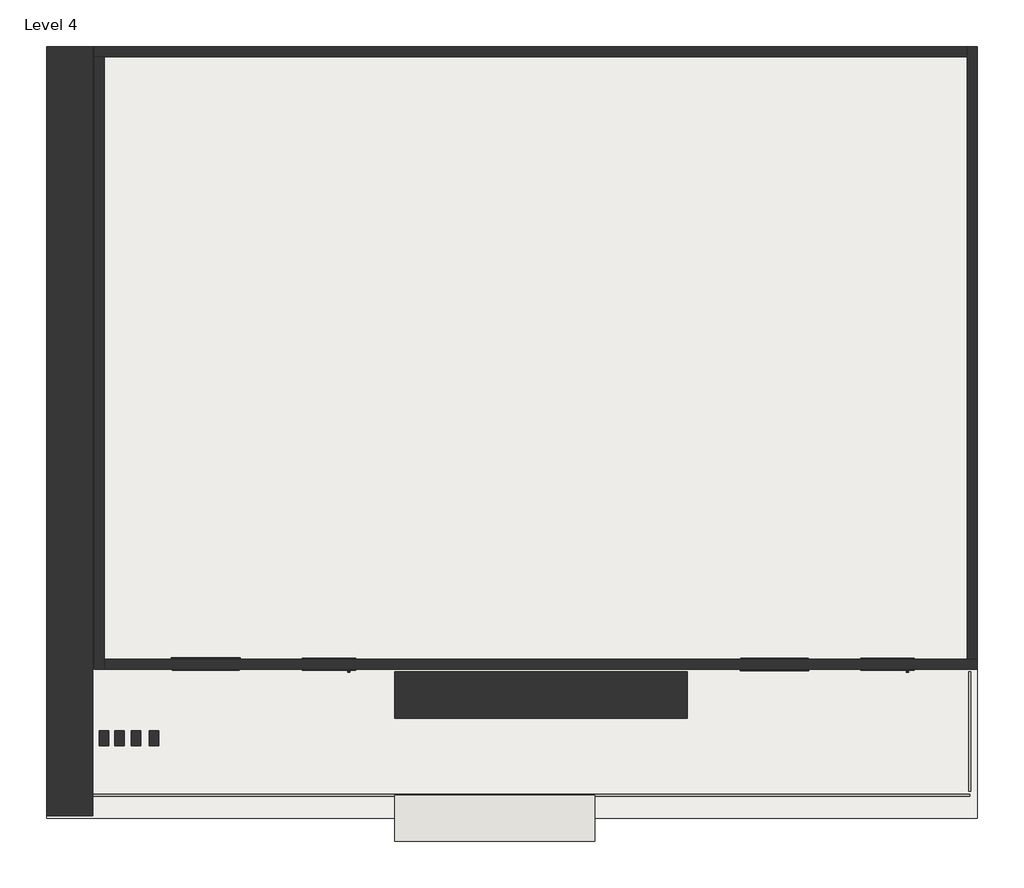
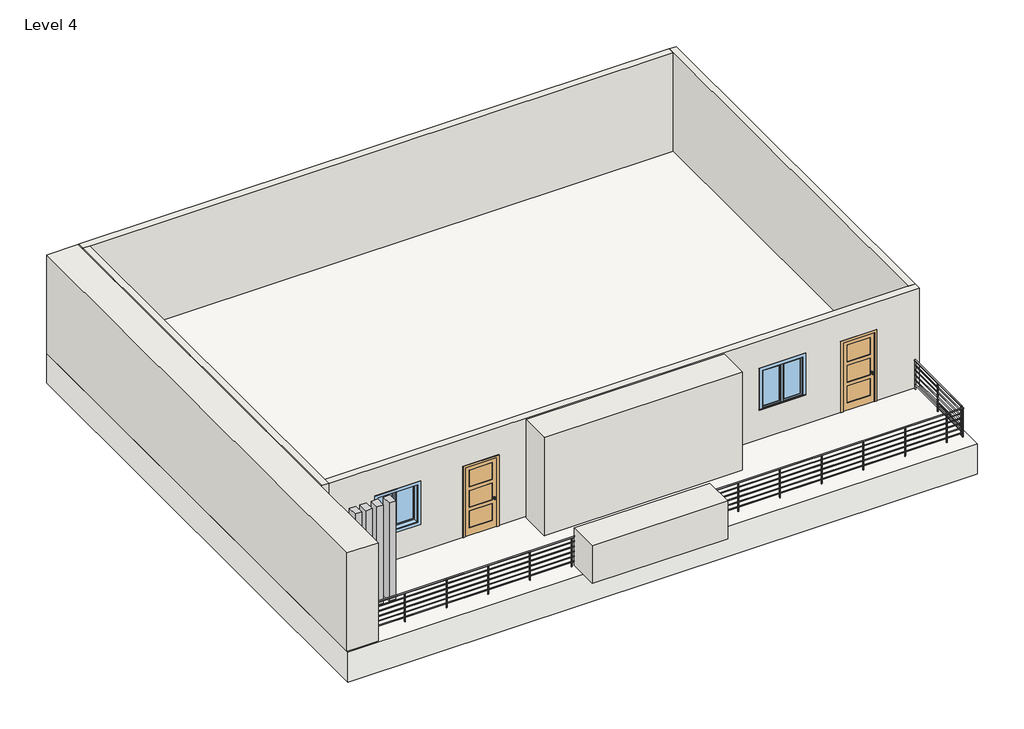
# One storey: 7 walls, 4 columns, 2 doors, 2 railings, 2 windows, 1 slab.
"""IFC4 building model written with IfcOpenShell, lengths in millimetres."""

from ifc_helpers import new_model, si_unit, point, frame, frame_2d, origin, place, context, project, spatial, polyline, circle_curve, trimmed, segment, composite_curve, outline, extrude, faceted_brep, transform, mapped, element, save
from components import wood_timber_column_8_x_12_853526f8, door_54d869bf, window_3a1167bf, window_0862ab64

model = new_model("IFC4")

# Units and contexts
model_context = context("Model", 3, world=origin())
ifc_project = project(units=[si_unit("LENGTHUNIT", "METRE", prefix="MILLI")], contexts=[model_context])

# Site, building, storey
site = spatial("IfcSite", under=ifc_project)
building = spatial("IfcBuilding", under=site)
storey = spatial("IfcBuildingStorey", under=building, Name="Level 4", Elevation=9144.0)

# Columns
placement = place(None, origin())
wood_timber_column_8_x_12_shape = wood_timber_column_8_x_12_853526f8(model_context)
element("IfcColumn", 1, ObjectType="Wood Timber Column : 8 x 12", at=placement, inside=storey, context=model_context, shape_type="MappedRepresentation", body=[
    mapped(wood_timber_column_8_x_12_shape, transform((-18270.7121948, 4590.8323495, 0.0), x_axis=(1.0, 0.0, 0.0), y_axis=(0.0, 1.0, 0.0), z_axis=(0.0, 0.0, 1.0))),
])
element("IfcColumn", 2, ObjectType="Wood Timber Column : 8 x 12", at=placement, inside=storey, context=model_context, shape_type="MappedRepresentation", body=[
    mapped(wood_timber_column_8_x_12_shape, transform((-18600.9121948, 4590.8323495, 0.0), x_axis=(1.0, 0.0, 0.0), y_axis=(0.0, 1.0, 0.0), z_axis=(0.0, 0.0, 1.0))),
])
element("IfcColumn", 3, ObjectType="Wood Timber Column : 8 x 12", at=placement, inside=storey, context=model_context, shape_type="MappedRepresentation", body=[
    mapped(wood_timber_column_8_x_12_shape, transform((-18905.7121948, 4590.8323495, 0.0), x_axis=(1.0, 0.0, 0.0), y_axis=(0.0, 1.0, 0.0), z_axis=(0.0, 0.0, 1.0))),
])
element("IfcColumn", 4, ObjectType="Wood Timber Column : 8 x 12", at=placement, inside=storey, context=model_context, shape_type="MappedRepresentation", body=[
    mapped(wood_timber_column_8_x_12_shape, transform((-17915.1121948, 4590.8323495, 0.0), x_axis=(1.0, 0.0, 0.0), y_axis=(0.0, 1.0, 0.0), z_axis=(0.0, 0.0, 1.0))),
])

# Doors
door_shape = door_54d869bf(model_context)
element("IfcDoor", 5, ObjectType="Door-Interior-Single-3_Panel_Vert-Wood : 36\" x 84\" 2", at=placement, inside=storey, context=model_context, shape_type="MappedRepresentation", body=[
    mapped(door_shape, transform((-3405.3621948, 6054.574368, 7844.0883406), x_axis=(-1.0, 0.0, 0.0), y_axis=(0.0, -1.0, 0.0), z_axis=(0.0, 0.0, 1.0))),
])
element("IfcDoor", 6, ObjectType="Door-Interior-Single-3_Panel_Vert-Wood : 36\" x 84\" 2", at=placement, inside=storey, context=model_context, shape_type="MappedRepresentation", body=[
    mapped(door_shape, transform((-14454.3621948, 6054.574368, 7844.0883406), x_axis=(-1.0, 0.0, 0.0), y_axis=(0.0, -1.0, 0.0), z_axis=(0.0, 0.0, 1.0))),
])

# Railings
element("IfcRailing", 7, ObjectType="Handrail - Pipe", at=placement, inside=storey, context=model_context, shape_type="SweptSolid", body=[
    extrude(outline(composite_curve([segment(trimmed(circle_curve(frame_2d((3466.949368, 8739.4383406)), 19.05), [point((3447.899368, 8739.4383406))], [point((3485.999368, 8739.4383406))], False, "CARTESIAN"), True, "CONTINUOUS"), segment(trimmed(circle_curve(frame_2d((3466.949368, 8739.4383406)), 19.05), [point((3485.999368, 8739.4383406))], [point((3447.899368, 8739.4383406))], False, "CARTESIAN"), True, "CONTINUOUS")], self_intersect=False)), frame((-19331.1621948, 0.0, 0.0), z_axis=(1.0, 0.0, 0.0), x_axis=(0.0, 1.0, 0.0)), (0.0, 0.0, 1.0), 17551.4),
    extrude(outline(composite_curve([segment(trimmed(circle_curve(frame_2d((3466.949368, 8593.3883406)), 12.7), [point((3479.649368, 8593.3883406))], [point((3454.249368, 8593.3883406))], False, "CARTESIAN"), True, "CONTINUOUS"), segment(trimmed(circle_curve(frame_2d((3466.949368, 8593.3883406)), 12.7), [point((3454.249368, 8593.3883406))], [point((3479.649368, 8593.3883406))], False, "CARTESIAN"), True, "CONTINUOUS")], self_intersect=False)), frame((-19331.1621948, 0.0, 0.0), z_axis=(1.0, 0.0, 0.0), x_axis=(0.0, 1.0, 0.0)), (0.0, 0.0, 1.0), 17551.4),
    extrude(outline(composite_curve([segment(trimmed(circle_curve(frame_2d((3466.949368, 8440.9883406)), 12.7), [point((3479.649368, 8440.9883406))], [point((3454.249368, 8440.9883406))], False, "CARTESIAN"), True, "CONTINUOUS"), segment(trimmed(circle_curve(frame_2d((3466.949368, 8440.9883406)), 12.7), [point((3454.249368, 8440.9883406))], [point((3479.649368, 8440.9883406))], False, "CARTESIAN"), True, "CONTINUOUS")], self_intersect=False)), frame((-19331.1621948, 0.0, 0.0), z_axis=(1.0, 0.0, 0.0), x_axis=(0.0, 1.0, 0.0)), (0.0, 0.0, 1.0), 17551.4),
    extrude(outline(composite_curve([segment(trimmed(circle_curve(frame_2d((3466.949368, 8288.5883406)), 12.7), [point((3479.649368, 8288.5883406))], [point((3454.249368, 8288.5883406))], False, "CARTESIAN"), True, "CONTINUOUS"), segment(trimmed(circle_curve(frame_2d((3466.949368, 8288.5883406)), 12.7), [point((3454.249368, 8288.5883406))], [point((3479.649368, 8288.5883406))], False, "CARTESIAN"), True, "CONTINUOUS")], self_intersect=False)), frame((-19331.1621948, 0.0, 0.0), z_axis=(1.0, 0.0, 0.0), x_axis=(0.0, 1.0, 0.0)), (0.0, 0.0, 1.0), 17551.4),
    extrude(outline(composite_curve([segment(trimmed(circle_curve(frame_2d((3466.949368, 8136.1883406)), 12.7), [point((3479.649368, 8136.1883406))], [point((3454.249368, 8136.1883406))], False, "CARTESIAN"), True, "CONTINUOUS"), segment(trimmed(circle_curve(frame_2d((3466.949368, 8136.1883406)), 12.7), [point((3454.249368, 8136.1883406))], [point((3479.649368, 8136.1883406))], False, "CARTESIAN"), True, "CONTINUOUS")], self_intersect=False)), frame((-19331.1621948, 0.0, 0.0), z_axis=(1.0, 0.0, 0.0), x_axis=(0.0, 1.0, 0.0)), (0.0, 0.0, 1.0), 17551.4),
    extrude(outline(composite_curve([segment(trimmed(circle_curve(frame_2d((3466.949368, 7983.7883406)), 12.7), [point((3479.649368, 7983.7883406))], [point((3454.249368, 7983.7883406))], False, "CARTESIAN"), True, "CONTINUOUS"), segment(trimmed(circle_curve(frame_2d((3466.949368, 7983.7883406)), 12.7), [point((3454.249368, 7983.7883406))], [point((3479.649368, 7983.7883406))], False, "CARTESIAN"), True, "CONTINUOUS")], self_intersect=False)), frame((-19331.1621948, 0.0, 0.0), z_axis=(1.0, 0.0, 0.0), x_axis=(0.0, 1.0, 0.0)), (0.0, 0.0, 1.0), 17551.4),
    extrude(outline(composite_curve([segment(trimmed(circle_curve(frame_2d((-2262.3621948, 3466.949368)), 12.7), [point((-2262.3621948, 3479.649368))], [point((-2262.3621948, 3454.249368))], False, "CARTESIAN"), True, "CONTINUOUS"), segment(trimmed(circle_curve(frame_2d((-2262.3621948, 3466.949368)), 12.7), [point((-2262.3621948, 3454.249368))], [point((-2262.3621948, 3479.649368))], False, "CARTESIAN"), True, "CONTINUOUS")], self_intersect=False)), frame((0.0, 0.0, 7844.0883406), z_axis=(0.0, 0.0, 1.0), x_axis=(1.0, 0.0, 0.0)), (0.0, 0.0, 1.0), 876.3),
    extrude(outline(composite_curve([segment(trimmed(circle_curve(frame_2d((-3481.5621948, 3466.949368)), 12.7), [point((-3481.5621948, 3479.649368))], [point((-3481.5621948, 3454.249368))], False, "CARTESIAN"), True, "CONTINUOUS"), segment(trimmed(circle_curve(frame_2d((-3481.5621948, 3466.949368)), 12.7), [point((-3481.5621948, 3454.249368))], [point((-3481.5621948, 3479.649368))], False, "CARTESIAN"), True, "CONTINUOUS")], self_intersect=False)), frame((0.0, 0.0, 7844.0883406), z_axis=(0.0, 0.0, 1.0), x_axis=(1.0, 0.0, 0.0)), (0.0, 0.0, 1.0), 876.3),
    extrude(outline(composite_curve([segment(trimmed(circle_curve(frame_2d((-4700.7621948, 3466.949368)), 12.7), [point((-4700.7621948, 3479.649368))], [point((-4700.7621948, 3454.249368))], False, "CARTESIAN"), True, "CONTINUOUS"), segment(trimmed(circle_curve(frame_2d((-4700.7621948, 3466.949368)), 12.7), [point((-4700.7621948, 3454.249368))], [point((-4700.7621948, 3479.649368))], False, "CARTESIAN"), True, "CONTINUOUS")], self_intersect=False)), frame((0.0, 0.0, 7844.0883406), z_axis=(0.0, 0.0, 1.0), x_axis=(1.0, 0.0, 0.0)), (0.0, 0.0, 1.0), 876.3),
    extrude(outline(composite_curve([segment(trimmed(circle_curve(frame_2d((-5919.9621948, 3466.949368)), 12.7), [point((-5919.9621948, 3479.649368))], [point((-5919.9621948, 3454.249368))], False, "CARTESIAN"), True, "CONTINUOUS"), segment(trimmed(circle_curve(frame_2d((-5919.9621948, 3466.949368)), 12.7), [point((-5919.9621948, 3454.249368))], [point((-5919.9621948, 3479.649368))], False, "CARTESIAN"), True, "CONTINUOUS")], self_intersect=False)), frame((0.0, 0.0, 7844.0883406), z_axis=(0.0, 0.0, 1.0), x_axis=(1.0, 0.0, 0.0)), (0.0, 0.0, 1.0), 876.3),
    extrude(outline(composite_curve([segment(trimmed(circle_curve(frame_2d((-7139.1621948, 3466.949368)), 12.7), [point((-7139.1621948, 3479.649368))], [point((-7139.1621948, 3454.249368))], False, "CARTESIAN"), True, "CONTINUOUS"), segment(trimmed(circle_curve(frame_2d((-7139.1621948, 3466.949368)), 12.7), [point((-7139.1621948, 3454.249368))], [point((-7139.1621948, 3479.649368))], False, "CARTESIAN"), True, "CONTINUOUS")], self_intersect=False)), frame((0.0, 0.0, 7844.0883406), z_axis=(0.0, 0.0, 1.0), x_axis=(1.0, 0.0, 0.0)), (0.0, 0.0, 1.0), 876.3),
    extrude(outline(composite_curve([segment(trimmed(circle_curve(frame_2d((-8358.3621948, 3466.949368)), 12.7), [point((-8358.3621948, 3479.649368))], [point((-8358.3621948, 3454.249368))], False, "CARTESIAN"), True, "CONTINUOUS"), segment(trimmed(circle_curve(frame_2d((-8358.3621948, 3466.949368)), 12.7), [point((-8358.3621948, 3454.249368))], [point((-8358.3621948, 3479.649368))], False, "CARTESIAN"), True, "CONTINUOUS")], self_intersect=False)), frame((0.0, 0.0, 7844.0883406), z_axis=(0.0, 0.0, 1.0), x_axis=(1.0, 0.0, 0.0)), (0.0, 0.0, 1.0), 876.3),
    extrude(outline(composite_curve([segment(trimmed(circle_curve(frame_2d((-9577.5621948, 3466.949368)), 12.7), [point((-9577.5621948, 3479.649368))], [point((-9577.5621948, 3454.249368))], False, "CARTESIAN"), True, "CONTINUOUS"), segment(trimmed(circle_curve(frame_2d((-9577.5621948, 3466.949368)), 12.7), [point((-9577.5621948, 3454.249368))], [point((-9577.5621948, 3479.649368))], False, "CARTESIAN"), True, "CONTINUOUS")], self_intersect=False)), frame((0.0, 0.0, 7844.0883406), z_axis=(0.0, 0.0, 1.0), x_axis=(1.0, 0.0, 0.0)), (0.0, 0.0, 1.0), 876.3),
    extrude(outline(composite_curve([segment(trimmed(circle_curve(frame_2d((-10796.7621948, 3466.949368)), 12.7), [point((-10796.7621948, 3479.649368))], [point((-10796.7621948, 3454.249368))], False, "CARTESIAN"), True, "CONTINUOUS"), segment(trimmed(circle_curve(frame_2d((-10796.7621948, 3466.949368)), 12.7), [point((-10796.7621948, 3454.249368))], [point((-10796.7621948, 3479.649368))], False, "CARTESIAN"), True, "CONTINUOUS")], self_intersect=False)), frame((0.0, 0.0, 7844.0883406), z_axis=(0.0, 0.0, 1.0), x_axis=(1.0, 0.0, 0.0)), (0.0, 0.0, 1.0), 876.3),
    extrude(outline(composite_curve([segment(trimmed(circle_curve(frame_2d((-12015.9621948, 3466.949368)), 12.7), [point((-12015.9621948, 3479.649368))], [point((-12015.9621948, 3454.249368))], False, "CARTESIAN"), True, "CONTINUOUS"), segment(trimmed(circle_curve(frame_2d((-12015.9621948, 3466.949368)), 12.7), [point((-12015.9621948, 3454.249368))], [point((-12015.9621948, 3479.649368))], False, "CARTESIAN"), True, "CONTINUOUS")], self_intersect=False)), frame((0.0, 0.0, 7844.0883406), z_axis=(0.0, 0.0, 1.0), x_axis=(1.0, 0.0, 0.0)), (0.0, 0.0, 1.0), 876.3),
    extrude(outline(composite_curve([segment(trimmed(circle_curve(frame_2d((-13235.1621948, 3466.949368)), 12.7), [point((-13235.1621948, 3479.649368))], [point((-13235.1621948, 3454.249368))], False, "CARTESIAN"), True, "CONTINUOUS"), segment(trimmed(circle_curve(frame_2d((-13235.1621948, 3466.949368)), 12.7), [point((-13235.1621948, 3454.249368))], [point((-13235.1621948, 3479.649368))], False, "CARTESIAN"), True, "CONTINUOUS")], self_intersect=False)), frame((0.0, 0.0, 7844.0883406), z_axis=(0.0, 0.0, 1.0), x_axis=(1.0, 0.0, 0.0)), (0.0, 0.0, 1.0), 876.3),
    extrude(outline(composite_curve([segment(trimmed(circle_curve(frame_2d((-14454.3621948, 3466.949368)), 12.7), [point((-14454.3621948, 3479.649368))], [point((-14454.3621948, 3454.249368))], False, "CARTESIAN"), True, "CONTINUOUS"), segment(trimmed(circle_curve(frame_2d((-14454.3621948, 3466.949368)), 12.7), [point((-14454.3621948, 3454.249368))], [point((-14454.3621948, 3479.649368))], False, "CARTESIAN"), True, "CONTINUOUS")], self_intersect=False)), frame((0.0, 0.0, 7844.0883406), z_axis=(0.0, 0.0, 1.0), x_axis=(1.0, 0.0, 0.0)), (0.0, 0.0, 1.0), 876.3),
    extrude(outline(composite_curve([segment(trimmed(circle_curve(frame_2d((-15673.5621948, 3466.949368)), 12.7), [point((-15673.5621948, 3479.649368))], [point((-15673.5621948, 3454.249368))], False, "CARTESIAN"), True, "CONTINUOUS"), segment(trimmed(circle_curve(frame_2d((-15673.5621948, 3466.949368)), 12.7), [point((-15673.5621948, 3454.249368))], [point((-15673.5621948, 3479.649368))], False, "CARTESIAN"), True, "CONTINUOUS")], self_intersect=False)), frame((0.0, 0.0, 7844.0883406), z_axis=(0.0, 0.0, 1.0), x_axis=(1.0, 0.0, 0.0)), (0.0, 0.0, 1.0), 876.3),
    extrude(outline(composite_curve([segment(trimmed(circle_curve(frame_2d((-16892.7621948, 3466.949368)), 12.7), [point((-16892.7621948, 3479.649368))], [point((-16892.7621948, 3454.249368))], False, "CARTESIAN"), True, "CONTINUOUS"), segment(trimmed(circle_curve(frame_2d((-16892.7621948, 3466.949368)), 12.7), [point((-16892.7621948, 3454.249368))], [point((-16892.7621948, 3479.649368))], False, "CARTESIAN"), True, "CONTINUOUS")], self_intersect=False)), frame((0.0, 0.0, 7844.0883406), z_axis=(0.0, 0.0, 1.0), x_axis=(1.0, 0.0, 0.0)), (0.0, 0.0, 1.0), 876.3),
    extrude(outline(composite_curve([segment(trimmed(circle_curve(frame_2d((-18111.9621948, 3466.949368)), 12.7), [point((-18111.9621948, 3479.649368))], [point((-18111.9621948, 3454.249368))], False, "CARTESIAN"), True, "CONTINUOUS"), segment(trimmed(circle_curve(frame_2d((-18111.9621948, 3466.949368)), 12.7), [point((-18111.9621948, 3454.249368))], [point((-18111.9621948, 3479.649368))], False, "CARTESIAN"), True, "CONTINUOUS")], self_intersect=False)), frame((0.0, 0.0, 7844.0883406), z_axis=(0.0, 0.0, 1.0), x_axis=(1.0, 0.0, 0.0)), (0.0, 0.0, 1.0), 876.3),
    extrude(outline(composite_curve([segment(trimmed(circle_curve(frame_2d((-1792.4621948, 3466.949368)), 12.7), [point((-1792.4621948, 3479.649368))], [point((-1792.4621948, 3454.249368))], False, "CARTESIAN"), True, "CONTINUOUS"), segment(trimmed(circle_curve(frame_2d((-1792.4621948, 3466.949368)), 12.7), [point((-1792.4621948, 3454.249368))], [point((-1792.4621948, 3479.649368))], False, "CARTESIAN"), True, "CONTINUOUS")], self_intersect=False)), frame((0.0, 0.0, 7844.0883406), z_axis=(0.0, 0.0, 1.0), x_axis=(1.0, 0.0, 0.0)), (0.0, 0.0, 1.0), 876.3),
    extrude(outline(composite_curve([segment(trimmed(circle_curve(frame_2d((-19318.4621948, 3466.949368)), 12.7), [point((-19318.4621948, 3479.649368))], [point((-19318.4621948, 3454.249368))], False, "CARTESIAN"), True, "CONTINUOUS"), segment(trimmed(circle_curve(frame_2d((-19318.4621948, 3466.949368)), 12.7), [point((-19318.4621948, 3454.249368))], [point((-19318.4621948, 3479.649368))], False, "CARTESIAN"), True, "CONTINUOUS")], self_intersect=False)), frame((0.0, 0.0, 7844.0883406), z_axis=(0.0, 0.0, 1.0), x_axis=(1.0, 0.0, 0.0)), (0.0, 0.0, 1.0), 876.3),
])
element("IfcRailing", 8, ObjectType="Handrail - Pipe", at=placement, inside=storey, context=model_context, shape_type="SweptSolid", body=[
    extrude(outline(composite_curve([segment(trimmed(circle_curve(frame_2d((8739.4383406, -1779.7621948)), 19.05), [point((8739.4383406, -1760.7121948))], [point((8739.4383406, -1798.8121948))], False, "CARTESIAN"), True, "CONTINUOUS"), segment(trimmed(circle_curve(frame_2d((8739.4383406, -1779.7621948)), 19.05), [point((8739.4383406, -1798.8121948))], [point((8739.4383406, -1760.7121948))], False, "CARTESIAN"), True, "CONTINUOUS")], self_intersect=False)), frame((0.0, 3543.149368, 0.0), z_axis=(0.0, 1.0, 0.0), x_axis=(0.0, 0.0, 1.0)), (0.0, 0.0, 1.0), 2362.2),
    extrude(outline(composite_curve([segment(trimmed(circle_curve(frame_2d((8593.3883406, -1779.7621948)), 12.7), [point((8593.3883406, -1792.4621948))], [point((8593.3883406, -1767.0621948))], False, "CARTESIAN"), True, "CONTINUOUS"), segment(trimmed(circle_curve(frame_2d((8593.3883406, -1779.7621948)), 12.7), [point((8593.3883406, -1767.0621948))], [point((8593.3883406, -1792.4621948))], False, "CARTESIAN"), True, "CONTINUOUS")], self_intersect=False)), frame((0.0, 3543.149368, 0.0), z_axis=(0.0, 1.0, 0.0), x_axis=(0.0, 0.0, 1.0)), (0.0, 0.0, 1.0), 2362.2),
    extrude(outline(composite_curve([segment(trimmed(circle_curve(frame_2d((8440.9883406, -1779.7621948)), 12.7), [point((8440.9883406, -1792.4621948))], [point((8440.9883406, -1767.0621948))], False, "CARTESIAN"), True, "CONTINUOUS"), segment(trimmed(circle_curve(frame_2d((8440.9883406, -1779.7621948)), 12.7), [point((8440.9883406, -1767.0621948))], [point((8440.9883406, -1792.4621948))], False, "CARTESIAN"), True, "CONTINUOUS")], self_intersect=False)), frame((0.0, 3543.149368, 0.0), z_axis=(0.0, 1.0, 0.0), x_axis=(0.0, 0.0, 1.0)), (0.0, 0.0, 1.0), 2362.2),
    extrude(outline(composite_curve([segment(trimmed(circle_curve(frame_2d((8288.5883406, -1779.7621948)), 12.7), [point((8288.5883406, -1792.4621948))], [point((8288.5883406, -1767.0621948))], False, "CARTESIAN"), True, "CONTINUOUS"), segment(trimmed(circle_curve(frame_2d((8288.5883406, -1779.7621948)), 12.7), [point((8288.5883406, -1767.0621948))], [point((8288.5883406, -1792.4621948))], False, "CARTESIAN"), True, "CONTINUOUS")], self_intersect=False)), frame((0.0, 3543.149368, 0.0), z_axis=(0.0, 1.0, 0.0), x_axis=(0.0, 0.0, 1.0)), (0.0, 0.0, 1.0), 2362.2),
    extrude(outline(composite_curve([segment(trimmed(circle_curve(frame_2d((8136.1883406, -1779.7621948)), 12.7), [point((8136.1883406, -1792.4621948))], [point((8136.1883406, -1767.0621948))], False, "CARTESIAN"), True, "CONTINUOUS"), segment(trimmed(circle_curve(frame_2d((8136.1883406, -1779.7621948)), 12.7), [point((8136.1883406, -1767.0621948))], [point((8136.1883406, -1792.4621948))], False, "CARTESIAN"), True, "CONTINUOUS")], self_intersect=False)), frame((0.0, 3543.149368, 0.0), z_axis=(0.0, 1.0, 0.0), x_axis=(0.0, 0.0, 1.0)), (0.0, 0.0, 1.0), 2362.2),
    extrude(outline(composite_curve([segment(trimmed(circle_curve(frame_2d((7983.7883406, -1779.7621948)), 12.7), [point((7983.7883406, -1792.4621948))], [point((7983.7883406, -1767.0621948))], False, "CARTESIAN"), True, "CONTINUOUS"), segment(trimmed(circle_curve(frame_2d((7983.7883406, -1779.7621948)), 12.7), [point((7983.7883406, -1767.0621948))], [point((7983.7883406, -1792.4621948))], False, "CARTESIAN"), True, "CONTINUOUS")], self_intersect=False)), frame((0.0, 3543.149368, 0.0), z_axis=(0.0, 1.0, 0.0), x_axis=(0.0, 0.0, 1.0)), (0.0, 0.0, 1.0), 2362.2),
    extrude(outline(composite_curve([segment(trimmed(circle_curve(frame_2d((-1779.7621948, 4762.349368)), 12.7), [point((-1792.4621948, 4762.349368))], [point((-1767.0621948, 4762.349368))], False, "CARTESIAN"), True, "CONTINUOUS"), segment(trimmed(circle_curve(frame_2d((-1779.7621948, 4762.349368)), 12.7), [point((-1767.0621948, 4762.349368))], [point((-1792.4621948, 4762.349368))], False, "CARTESIAN"), True, "CONTINUOUS")], self_intersect=False)), frame((0.0, 0.0, 7844.0883406), z_axis=(0.0, 0.0, 1.0), x_axis=(1.0, 0.0, 0.0)), (0.0, 0.0, 1.0), 876.3),
    extrude(outline(composite_curve([segment(trimmed(circle_curve(frame_2d((-1779.7621948, 5892.649368)), 12.7), [point((-1792.4621948, 5892.649368))], [point((-1767.0621948, 5892.649368))], False, "CARTESIAN"), True, "CONTINUOUS"), segment(trimmed(circle_curve(frame_2d((-1779.7621948, 5892.649368)), 12.7), [point((-1767.0621948, 5892.649368))], [point((-1792.4621948, 5892.649368))], False, "CARTESIAN"), True, "CONTINUOUS")], self_intersect=False)), frame((0.0, 0.0, 7844.0883406), z_axis=(0.0, 0.0, 1.0), x_axis=(1.0, 0.0, 0.0)), (0.0, 0.0, 1.0), 876.3),
    extrude(outline(composite_curve([segment(trimmed(circle_curve(frame_2d((-1779.7621948, 3555.849368)), 12.7), [point((-1792.4621948, 3555.849368))], [point((-1767.0621948, 3555.849368))], False, "CARTESIAN"), True, "CONTINUOUS"), segment(trimmed(circle_curve(frame_2d((-1779.7621948, 3555.849368)), 12.7), [point((-1767.0621948, 3555.849368))], [point((-1792.4621948, 3555.849368))], False, "CARTESIAN"), True, "CONTINUOUS")], self_intersect=False)), frame((0.0, 0.0, 7844.0883406), z_axis=(0.0, 0.0, 1.0), x_axis=(1.0, 0.0, 0.0)), (0.0, 0.0, 1.0), 876.3),
])

# Slab
element("IfcSlab", 9, ObjectType="Generic - 3'", at=placement, inside=storey, context=model_context, shape_type="SweptSolid", body=[
    extrude(outline(polyline([(-1627.3621948, 18275.149368), (-1627.3621948, 3009.749368), (-20042.3621948, 3009.749368), (-20042.3621948, 18275.149368), (-1627.3621948, 18275.149368)])), frame((0.0, 0.0, 6929.6883406), z_axis=(0.0, 0.0, 1.0), x_axis=(1.0, 0.0, 0.0)), (0.0, 0.0, 1.0), 914.4),
])

# Walls
element("IfcWall", 10, ObjectType="Generic - 3' 2", at=placement, inside=storey, context=model_context, shape_type="SweptSolid", body=[
    extrude(outline(polyline([(-7367.7621948, 4990.949368), (-13158.9621948, 4990.949368), (-13158.9621948, 5905.349368), (-7367.7621948, 5905.349368), (-7367.7621948, 4990.949368)])), frame((0.0, 0.0, 7844.0883406), z_axis=(0.0, 0.0, 1.0), x_axis=(1.0, 0.0, 0.0)), (0.0, 0.0, 1.0), 3048.0),
])
element("IfcWall", 11, ObjectType="Generic - 3' 4", at=placement, inside=storey, context=model_context, shape_type="SweptSolid", body=[
    extrude(outline(polyline([(-9196.5621948, 2552.549368), (-13158.9621948, 2552.549368), (-13158.9621948, 3466.949368), (-9196.5621948, 3466.949368), (-9196.5621948, 2552.549368)])), frame((0.0, 0.0, 7844.0883406), z_axis=(0.0, 0.0, 1.0), x_axis=(1.0, 0.0, 0.0)), (0.0, 0.0, 1.0), 1165.3811612),
])
element("IfcWall", 12, ObjectType="Generic - 3' 4", at=placement, inside=storey, context=model_context, shape_type="SweptSolid", body=[
    extrude(outline(polyline([(-20042.3621948, 3060.549368), (-20042.3621948, 18275.149368), (-19127.9621948, 18275.149368), (-19127.9621948, 3060.549368), (-20042.3621948, 3060.549368)])), frame((0.0, 0.0, 7844.0883406), z_axis=(0.0, 0.0, 1.0), x_axis=(1.0, 0.0, 0.0)), (0.0, 0.0, 1.0), 3048.0),
])
element("IfcWall", 13, ObjectType="Generic - 8\"", at=placement, inside=storey, context=model_context, shape_type="Brep", body=[
    faceted_brep([(-19102.5621948, 18071.949368, 7844.0883406), (-18899.3621948, 18071.949368, 7844.0883406), (-1830.5621948, 18071.949368, 7844.0883406), (-1830.5621948, 18071.949368, 10892.0883406), (-18899.3621948, 18071.949368, 10892.0883406), (-19102.5621948, 18071.949368, 10892.0883406), (-19102.5621948, 18275.149368, 7844.0883406), (-19102.5621948, 18275.149368, 10892.0883406), (-1830.5621948, 18275.149368, 10892.0883406), (-1830.5621948, 18275.149368, 7844.0883406)], [[[0, 1, 2, 3, 4, 5]], [[6, 7, 8, 9]], [[2, 1, 0, 6, 9]], [[5, 4, 3, 8, 7]], [[0, 5, 7, 6]], [[3, 2, 9, 8]]]),
])
element("IfcWall", 14, ObjectType="Generic - 8\"", at=placement, inside=storey, context=model_context, shape_type="Brep", body=[
    faceted_brep([(-18899.3621948, 6159.349368, 10892.0883406), (-1830.5621948, 6159.349368, 10892.0883406), (-1627.3621948, 6159.349368, 10892.0883406), (-1627.3621948, 6159.349368, 7844.0883406), (-1830.5621948, 6159.349368, 7844.0883406), (-2922.7621948, 6159.349368, 7844.0883406), (-2922.7621948, 6159.349368, 10003.0883406), (-3887.9621948, 6159.349368, 10003.0883406), (-3887.9621948, 6159.349368, 7844.0883406), (-13971.7621948, 6159.349368, 7844.0883406), (-13971.7621948, 6159.349368, 10003.0883406), (-14936.9621948, 6159.349368, 10003.0883406), (-14936.9621948, 6159.349368, 7844.0883406), (-18899.3621948, 6159.349368, 7844.0883406), (-17502.3621948, 6159.349368, 9977.6883406), (-17502.3621948, 6159.349368, 8758.4883406), (-16283.1621948, 6159.349368, 8758.4883406), (-16283.1621948, 6159.349368, 9977.6883406), (-6250.1621948, 6159.349368, 9977.6883406), (-6250.1621948, 6159.349368, 8758.4883406), (-5030.9621948, 6159.349368, 8758.4883406), (-5030.9621948, 6159.349368, 9977.6883406), (-1627.3621948, 5956.149368, 10892.0883406), (-18899.3621948, 5956.149368, 10892.0883406), (-18899.3621948, 5956.149368, 7844.0883406), (-14936.9621948, 5956.149368, 7844.0883406), (-14936.9621948, 5956.149368, 10003.0883406), (-13971.7621948, 5956.149368, 10003.0883406), (-13971.7621948, 5956.149368, 7844.0883406), (-3887.9621948, 5956.149368, 7844.0883406), (-3887.9621948, 5956.149368, 10003.0883406), (-2922.7621948, 5956.149368, 10003.0883406), (-2922.7621948, 5956.149368, 7844.0883406), (-1627.3621948, 5956.149368, 7844.0883406), (-17502.3621948, 5956.149368, 9977.6883406), (-16283.1621948, 5956.149368, 9977.6883406), (-16283.1621948, 5956.149368, 8758.4883406), (-17502.3621948, 5956.149368, 8758.4883406), (-6250.1621948, 5956.149368, 9977.6883406), (-5030.9621948, 5956.149368, 9977.6883406), (-5030.9621948, 5956.149368, 8758.4883406), (-6250.1621948, 5956.149368, 8758.4883406)], [[[0, 1, 2, 3, 4, 5, 6, 7, 8, 9, 10, 11, 12, 13], [14, 15, 16, 17], [18, 19, 20, 21]], [[22, 23, 24, 25, 26, 27, 28, 29, 30, 31, 32, 33], [34, 35, 36, 37], [38, 39, 40, 41]], [[3, 33, 32, 5, 4]], [[8, 29, 28, 9]], [[24, 13, 12, 25]], [[2, 1, 0, 23, 22]], [[3, 2, 22, 33]], [[7, 30, 29, 8]], [[30, 7, 6, 31]], [[31, 6, 5, 32]], [[11, 26, 25, 12]], [[26, 11, 10, 27]], [[27, 10, 9, 28]], [[15, 14, 34, 37]], [[16, 15, 37, 36]], [[17, 16, 36, 35]], [[14, 17, 35, 34]], [[19, 18, 38, 41]], [[20, 19, 41, 40]], [[21, 20, 40, 39]], [[18, 21, 39, 38]], [[0, 13, 24, 23]]]),
])
element("IfcWall", 15, ObjectType="Generic - 8\"", at=placement, inside=storey, context=model_context, shape_type="Brep", body=[
    faceted_brep([(-1830.5621948, 18275.149368, 7844.0883406), (-1830.5621948, 18071.949368, 7844.0883406), (-1830.5621948, 6159.349368, 7844.0883406), (-1830.5621948, 6159.349368, 10892.0883406), (-1830.5621948, 18071.949368, 10892.0883406), (-1830.5621948, 18275.149368, 10892.0883406), (-1627.3621948, 18275.149368, 7844.0883406), (-1627.3621948, 18275.149368, 10892.0883406), (-1627.3621948, 6159.349368, 10892.0883406), (-1627.3621948, 6159.349368, 7844.0883406)], [[[0, 1, 2, 3, 4, 5]], [[6, 7, 8, 9]], [[2, 1, 0, 6, 9]], [[5, 4, 3, 8, 7]], [[0, 5, 7, 6]], [[3, 2, 9, 8]]]),
])
element("IfcWall", 16, ObjectType="Generic - 8\"", at=placement, inside=storey, context=model_context, shape_type="Brep", body=[
    faceted_brep([(-18899.3621948, 5956.149368, 7844.0883406), (-18899.3621948, 6159.349368, 7844.0883406), (-18899.3621948, 18071.949368, 7844.0883406), (-18899.3621948, 18071.949368, 10892.0883406), (-18899.3621948, 6159.349368, 10892.0883406), (-18899.3621948, 5956.149368, 10892.0883406), (-19102.5621948, 5956.149368, 7844.0883406), (-19102.5621948, 5956.149368, 10892.0883406), (-19102.5621948, 18071.949368, 10892.0883406), (-19102.5621948, 18071.949368, 7844.0883406)], [[[0, 1, 2, 3, 4, 5]], [[6, 7, 8, 9]], [[2, 1, 0, 6, 9]], [[5, 4, 3, 8, 7]], [[3, 2, 9, 8]], [[0, 5, 7, 6]]]),
])

# Windows
window_shape = window_3a1167bf(model_context)
element("IfcWindow", 17, ObjectType="Casement Dbl with Trim : 48\" x 48\"", at=placement, inside=storey, context=model_context, shape_type="MappedRepresentation", body=[
    mapped(window_shape, transform((-16892.7621948, 6038.699368, 7844.0883406), x_axis=(-1.0, 0.0, 0.0), y_axis=(0.0, -1.0, 0.0), z_axis=(0.0, 0.0, 1.0))),
])
window_2_shape = window_0862ab64(model_context)
element("IfcWindow", 18, ObjectType="Casement Dbl with Trim : 48\" x 48\" 2", at=placement, inside=storey, context=model_context, shape_type="MappedRepresentation", body=[
    mapped(window_2_shape, transform((-5640.5621948, 6076.799368, 7844.0883406), x_axis=(-1.0, 0.0, 0.0), y_axis=(0.0, -1.0, 0.0), z_axis=(0.0, 0.0, 1.0))),
])

save(model, "model.ifc")

# Revit data of these elements
# Type "Wood Timber Column : 8 x 12"
#   Assembly Code = "B1010200"
#   Depth = 0' - 11 1/2"
#   Width = 0' - 7 1/2"
#   Material = Softwood, Lumber
# Type "Door-Interior-Single-3_Panel_Vert-Wood : 36\" x 84\" 2"
#   Type Mark = "11"
#   Assembly Code = "C1020300"
#   Analytic Construction = "Wooden"
#   Top Rail = 0' - 4 11/16"
#   Thickness = 0' - 1 3/8"
#   Thermal Resistance (R) = 2.5876 (h·ft²·°F)/BTU
#   Swing Angle [instance default] = 90.00°
#   Stiles = 0' - 4 3/4"
#   Rough Width = 3' - 2"
#   Rough Height = 7' - 1"
#   Intermediate Rail = 0' - 4 1/2"
#   Height = 7' - 0"
#   Width = 3' - 0"
#   Heat Transfer Coefficient (U) = 0.3865 BTU/(h·ft²·°F)
#   Bottom Rail = 0' - 9 1/8"
#   Trim Material = Cherry
#   Panel Material = Door - Panel
#   Frame Material = Door - Panel
#   Door Handle Material = Aluminum
#   Visual Light Transmittance = 0
#   Solar Heat Gain Coefficient = 0
#   Wall Closure = (empty or 0)
#   Function = (empty or 0)
# Type "Handrail - Pipe"
#   Assembly Code = "C2010400"
#   built-in parameter 1008612 = 0.0416667 (stored number, unit not read)
#   built-in parameter 1008611 = 0.0833333 (stored number, unit not read)
#   built-in parameter 1008609 = 4 (stored number, unit not read)
#   built-in parameter 1008604 = 0.166667 (stored number, unit not read)
#   built-in parameter 1008603 = 0.166667 (stored number, unit not read)
#   Railing Height = 3' - 0"
#   built-in parameter 1008630 = 2
#   built-in parameter 1008610 = 1
#   built-in parameter 1008605 = 1
#   built-in parameter 1008618 = Baluster - Round : 1"
# Type "Generic - 3'"
#   Assembly Code = "B1010"
#   Function = 0
#   Layers, outside or top first: 3' - 0" "Parking Stripe" (function 1)
# Type "Generic - 3' 2"
#   Assembly Code = "B2010"
#   Layers, outside or top first: 3' - 0" "Asphalt Shingle" (function 1)
# Type "Generic - 3' 4"
#   Assembly Code = "B2010"
#   Layers, outside or top first: 3' - 0" "Parking Stripe" (function 1)
# Type "Generic - 8\""
#   Assembly Code = "B2010"
#   Layers, outside or top first: 0' - 8" "Paint - Sienna" (function 1)
# Type "Casement Dbl with Trim : 48\" x 48\""
#   Type Mark = "10"
#   Construction Type Id = "GSP4R"
#   Assembly Code = "B2020100"
#   Analytic Construction = "1/8 in Pilkington single glazing"
#   Visual Light Transmittance = 0.9
#   Thermal Resistance (R) = 1.53941 (h·ft²·°F)/BTU
#   Solar Heat Gain Coefficient = 0.78
#   Heat Transfer Coefficient (U) = 0.6496 BTU/(h·ft²·°F)
#   Height = 4' - 0"
#   Default Sill Height = 3' - 0"
#   Trim Projection - Ext. = 0' - 0 1/2"
#   Trim Projection - Int. = 0' - 0 3/4"
#   Trim Width - Exterior = 0' - 3 1/2"
#   Trim Width - Interior = 0' - 3 1/2"
#   Width = 4' - 0"
#   Window Inset = 0' - 0 3/4"
#   Define Thermal Properties by = 1
#   Glass Pane Material = Glass
#   Sash Material = Sash
#   Trim Exterior Material = Trim
#   Trim Interior Material = Trim
#   Wall Closure = (empty or 0)
# Type "Casement Dbl with Trim : 48\" x 48\" 2"
#   Type Mark = "13"
#   Construction Type Id = "GSP4R"
#   Assembly Code = "B2020100"
#   Analytic Construction = "1/8 in Pilkington single glazing"
#   Visual Light Transmittance = 0.9
#   Thermal Resistance (R) = 1.53941 (h·ft²·°F)/BTU
#   Solar Heat Gain Coefficient = 0.78
#   Heat Transfer Coefficient (U) = 0.6496 BTU/(h·ft²·°F)
#   Height = 4' - 0"
#   Default Sill Height = 3' - 0"
#   Trim Projection - Ext. = 0' - 0 1/2"
#   Trim Projection - Int. = 0' - 0 3/4"
#   Trim Width - Exterior = 0' - 3 1/2"
#   Trim Width - Interior = 0' - 3 1/2"
#   Width = 4' - 0"
#   Window Inset = 0' - 0 3/4"
#   Define Thermal Properties by = 1
#   Glass Pane Material = Glass, Clear Glazing
#   Sash Material = Copper
#   Trim Exterior Material = Earth
#   Trim Interior Material = Earth
#   Wall Closure = (empty or 0)
# Elements 1, 2, 3, 4 (IfcColumn, "Wood Timber Column : 8 x 12")
#   Phase Created = New Construction
#   Materials on its faces: "Softwood, Lumber"
# Elements 5, 6 (IfcDoor, "Door-Interior-Single-3_Panel_Vert-Wood : 36\" x 84\" 2")
#   Swing Angle = 90.00°
#   Phase Created = New Construction
#   Materials on its faces: "Door - Panel", "Aluminum", "Cherry"
# Elements 7, 8 (IfcRailing, "Handrail - Pipe")
#   built-in parameter 1008621 = -4.2648 (stored number, unit not read)
#   Phase Created = New Construction
# Element 9 (IfcSlab, "Generic - 3'")
#   Height Offset From Level = -4' - 3.17762"
#   Phase Created = New Construction
#   Materials on its faces: "Parking Stripe"
# Element 10 (IfcWall, "Generic - 3' 2")
#   built-in parameter 1001111 = -4' - 3.17762"
#   Top Offset = 0' - 0"
#   Base Offset = -4' - 3.17762"
#   Unconnected Height = 10' - 0"
#   wall height = 10' - 0"
#   Phase Created = New Construction
#   Base Constraint = Level 4
#   Materials on its faces: "Asphalt Shingle"
# Element 11 (IfcWall, "Generic - 3' 4")
#   built-in parameter 1001111 = -4' - 3.17762"
#   Top Offset = 0' - 0"
#   Base Offset = -4' - 3.17762"
#   Unconnected Height = 3' - 9.88115"
#   wall height = 3' - 9.88115"
#   Phase Created = New Construction
#   Base Constraint = Level 4
#   Materials on its faces: "Parking Stripe"
# Element 12 (IfcWall, "Generic - 3' 4")
#   built-in parameter 1001111 = -4' - 3.17762"
#   Top Offset = 0' - 0"
#   Base Offset = -4' - 3.17762"
#   Unconnected Height = 10' - 0"
#   wall height = 10' - 0"
#   Phase Created = New Construction
#   Base Constraint = Level 4
#   Materials on its faces: "Parking Stripe"
# Elements 13, 14, 15, 16 (IfcWall, "Generic - 8\"")
#   built-in parameter 1001111 = -4' - 3.17762"
#   Top Offset = 0' - 0"
#   Base Offset = -4' - 3.17762"
#   Unconnected Height = 10' - 0"
#   wall height = 10' - 0"
#   Phase Created = New Construction
#   Base Constraint = Level 4
#   Materials on its faces: "Paint - Sienna"
# Element 17 (IfcWindow, "Casement Dbl with Trim : 48\" x 48\"")
#   Mark = "8"
#   Phase Created = New Construction
#   Materials on its faces: "Sash", "Trim", "Glass"
# Element 18 (IfcWindow, "Casement Dbl with Trim : 48\" x 48\" 2")
#   Mark = "9"
#   Phase Created = New Construction
#   Materials on its faces: "Copper", "Earth", "Glass, Clear Glazing"
# Materials
#   "Softwood, Lumber": class "Wood", colour RGB 223 192 134, transparency 0, Description = "Pinus Echinata", Cost = 0
#   "Cherry": class "Wood", colour RGB 226 177 128, transparency 0, Description = "Prunus Serotina", Cost = 0
#   "Door - Panel": class "Wood", colour RGB 210 159 95, transparency 0
#   "Aluminum": class "Metal", colour RGB 247 247 247, transparency 0, Description = "Aluminum 6061", Cost = 0
#   "Parking Stripe": class "Paint", colour RGB 255 221 187, transparency 0, Cost = 0
#   "Asphalt Shingle": class "Generic", colour RGB 155 155 155, transparency 0, Description = "Asphalt roofing shingle", Cost = 0
#   "Paint - Sienna": colour RGB 255 255 255, transparency 0, Cost = 0
#   "Glass": class "Glass", colour RGB 0 128 192, transparency 0.75, Description = "Soda Lime Glass", Cost = 0
#   "Sash": class "Wood", colour RGB 224 178 126, transparency 0
#   "Trim": class "Wood", colour RGB 224 178 126, transparency 0
#   "Glass, Clear Glazing": class "Glass", colour RGB 0 128 192, transparency 0.75, Description = "Clear glazing", Cost = 0
#   "Copper": class "Metal", colour RGB 0 0 0, transparency 0, Description = "Copper, matte finish", Cost = 0
#   "Earth": class "Generic", colour RGB 97 75 62, transparency 0, Description = "Soil", Cost = 0
